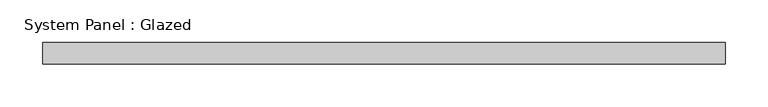
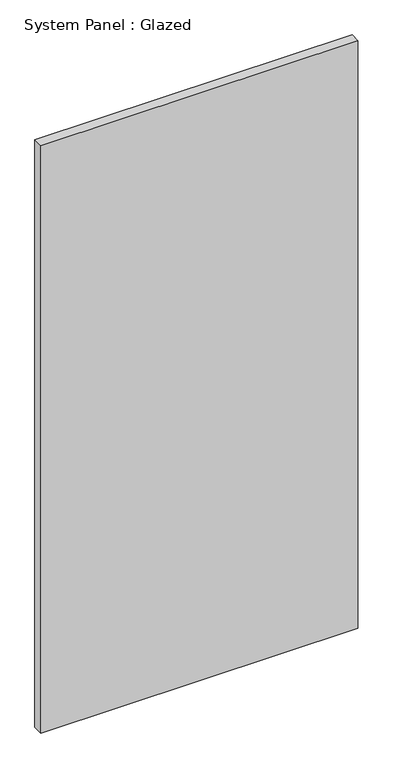
"""IFC4 building model written with IfcOpenShell, lengths in millimetres: plate geometry, System Panel : Glazed."""

from ifc_helpers import new_model, si_unit, origin, origin_with_axes, place, context, project, spatial, polyline, outline, extrude, source, transform, mapped, element, save


def system_panel_glazed_fe3e992a(model_context):
    return source(origin(), model_context, "Body", "SweptSolid", [
        extrude(outline(polyline([(400.05, 19.05), (-400.05, 19.05), (-400.05, 44.45), (400.05, 44.45), (400.05, 19.05)])), origin_with_axes(), (0.0, 0.0, 1.0), 1566.6943888),
    ])


if __name__ == "__main__":
    model = new_model("IFC4")
    model_context = context("Model", 3, world=origin())
    ifc_project = project(units=[si_unit("LENGTHUNIT", "METRE", prefix="MILLI")], contexts=[model_context])
    site = spatial("IfcSite", under=ifc_project)
    building = spatial("IfcBuilding", under=site)
    placement = place(None, origin())
    system_panel_glazed_shape = system_panel_glazed_fe3e992a(model_context)
    element("IfcPlate", 1, ObjectType="System Panel : Glazed", at=placement, inside=building, context=model_context, shape_type="MappedRepresentation", body=[
        mapped(system_panel_glazed_shape, transform((0.0, 0.0, 0.0), x_axis=(1.0, 0.0, 0.0), y_axis=(0.0, 1.0, 0.0), z_axis=(0.0, 0.0, 1.0))),
    ])
    save(model, "model.ifc")

# Revit data of these elements
# Type "System Panel : Glazed"
#   Construction Type Id = "GSP4R"
#   Analytic Construction = "1/8 in Pilkington single glazing"
#   Visual Light Transmittance = 0.9
#   Solar Heat Gain Coefficient = 0.86
#   Heat Transfer Coefficient (U) = 1.18115 BTU/(h·ft²·°F)
#   Define Thermal Properties by = 1
# Element 1 (IfcPlate, "System Panel : Glazed")
#   Materials on its faces: "Glass"
# Materials
#   "Glass": class "Glass", colour RGB 0 128 192, transparency 0.75, Description = "Soda Lime Glass", Cost = 0
